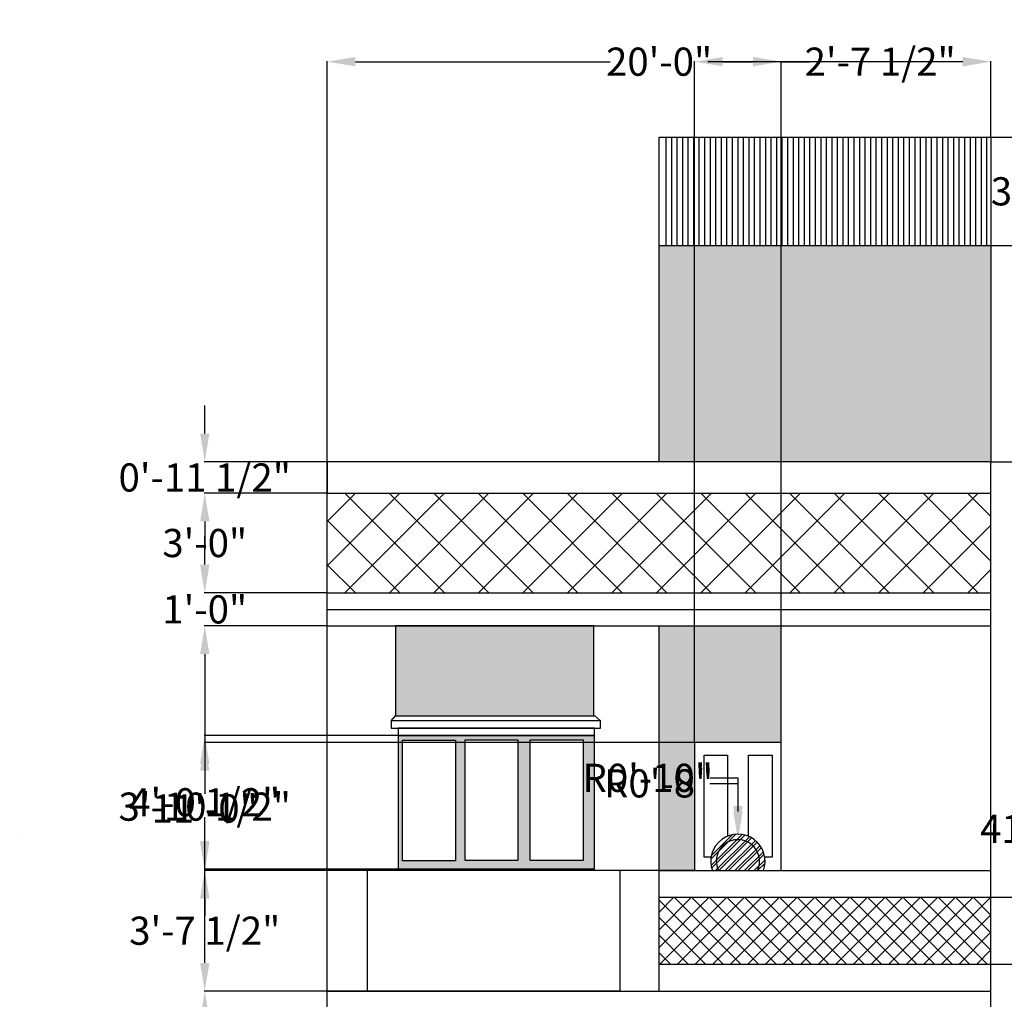
# Model space of a CAD drawing. Units: inches. Extents: x 21 to 3450, y 4 to 2137.
# Tile 6 of 14: x 2075 to 2431, y 1783 to 2137. Entities that reach past the tile are written whole.
import ezdxf

# ---------------------------------------------------------------- set-up
doc = ezdxf.new("R2010")
doc.units = ezdxf.units.IN
doc.header["$MEASUREMENT"] = 0
for name, color, linetype, lineweight in [('A-ANNO-DIMS', 2, 'Continuous', 18), ('A-ELEV', 7, 'Continuous', 25), ('A-ELEV-PATT', 8, 'Continuous', 13)]:
    doc.layers.add(name, color=color, linetype=linetype, lineweight=lineweight)
doc.styles.get("Standard").update_dxf_attribs({"font": 'arial.ttf'})
doc.dimstyles.get("Standard").update_dxf_attribs({"dimtxt": 10.18, "dimasz": 10.18, "dimexe": 0.18, "dimexo": 0.0625, "dimgap": 0.09, "dimtad": 0, "dimtih": 1, "dimtoh": 1, "dimdec": 0, "dimzin": 0, "dimdsep": 46, "dimlunit": 3, "dimtxsty": 'Standard', "dimcen": 0.09, "dimadec": 0, "dimazin": 0, "dimtfac": 1, "dimtdec": 0, "dimtofl": 0, "dimtmove": 0, "dimatfit": 3, "dimfxl": 1, "dimtolj": 1, "dimtzin": 0, "dimarcsym": 0})

# ---------------------------------------------------------------- blocks, each defined once
blk = doc.blocks.new('*D151')
at = {"layer": 'A-ANNO-DIMS', "color": 0, "lineweight": -2, "transparency": 16777216}
for p, q in [((2186.18, 1977.55), (2186.18, 2122.33)), ((2196.36, 2122.15), (2288.52, 2122.15)), ((2416, 2122.15), (2323.85, 2122.15)), ((2426.18, 2094.96), (2426.18, 2122.33))]:
    blk.add_line(p, q, dxfattribs=at)
at = {"layer": 'A-ANNO-DIMS', "color": 0, "transparency": 16777216}
for points in [[(2196.36, 2123.85), (2196.36, 2120.46), (2186.18, 2122.15)], [(2416, 2123.85), (2416, 2120.46), (2426.18, 2122.15)]]:
    blk.add_solid(points, dxfattribs=at)
at = {"layer": 'Defpoints', "color": 0, "transparency": 16777216}
for p in [(2426.18, 2122.15), (2426.18, 2094.9), (2186.18, 1977.49)]:
    blk.add_point(p, dxfattribs=at)
at = {"layer": 'A-ANNO-DIMS', "color": 0, "transparency": 16777216, "insert": (2306.18, 2122.15), "char_height": 10.18, "attachment_point": 5}
blk.add_mtext('\\A1;20\'-0"', dxfattribs=at)
blk = doc.blocks.new('*D152')
at = {"layer": 'A-ANNO-DIMS', "color": 0, "lineweight": -2, "transparency": 16777216}
for p, q in [((2426.25, 2094.9), (2453.61, 2094.9)), ((2453.43, 2084.72), (2453.43, 1850.06)), ((2453.43, 1604.7), (2453.43, 1839.36)), ((2426.25, 1594.52), (2453.61, 1594.52))]:
    blk.add_line(p, q, dxfattribs=at)
at = {"layer": 'A-ANNO-DIMS', "color": 0, "transparency": 16777216}
for points in [[(2451.74, 2084.72), (2455.13, 2084.72), (2453.43, 2094.9)], [(2451.74, 1604.7), (2455.13, 1604.7), (2453.43, 1594.52)]]:
    blk.add_solid(points, dxfattribs=at)
at = {"layer": 'Defpoints', "color": 0, "transparency": 16777216}
for p in [(2426.18, 2094.9), (2453.43, 2094.9), (2426.18, 1594.52)]:
    blk.add_point(p, dxfattribs=at)
at = {"layer": 'A-ANNO-DIMS', "color": 0, "transparency": 16777216, "insert": (2453.43, 1844.71), "char_height": 10.18, "attachment_point": 5}
blk.add_mtext('\\A1;41\'-8 1/2"', dxfattribs=at)
blk = doc.blocks.new('*D154')
at = {"layer": 'A-ANNO-DIMS', "color": 0, "lineweight": -2, "transparency": 16777216}
for p, q in [((2186.12, 1786.08), (2141.7, 1786.08)), ((2141.88, 1775.9), (2141.88, 1716.37)), ((2141.88, 1646.26), (2141.88, 1705.79)), ((2186.12, 1636.08), (2141.7, 1636.08))]:
    blk.add_line(p, q, dxfattribs=at)
at = {"layer": 'A-ANNO-DIMS', "color": 0, "transparency": 16777216}
for points in [[(2140.19, 1775.9), (2143.58, 1775.9), (2141.88, 1786.08)], [(2140.19, 1646.26), (2143.58, 1646.26), (2141.88, 1636.08)]]:
    blk.add_solid(points, dxfattribs=at)
at = {"layer": 'Defpoints', "color": 0, "transparency": 16777216}
for p in [(2141.88, 1786.08), (2186.18, 1786.08), (2186.18, 1636.08)]:
    blk.add_point(p, dxfattribs=at)
at = {"layer": 'A-ANNO-DIMS', "color": 0, "transparency": 16777216, "insert": (2141.88, 1711.08), "char_height": 10.18, "attachment_point": 5}
blk.add_mtext('\\A1;12\'-6"', dxfattribs=at)
blk = doc.blocks.new('*D155')
at = {"layer": 'A-ANNO-DIMS', "color": 0, "lineweight": -2, "transparency": 16777216}
for p, q in [((2186.12, 1918.08), (2141.7, 1918.08)), ((2141.88, 1907.9), (2141.88, 1857.37)), ((2141.88, 1796.26), (2141.88, 1846.79)), ((2186.12, 1786.08), (2141.7, 1786.08))]:
    blk.add_line(p, q, dxfattribs=at)
at = {"layer": 'A-ANNO-DIMS', "color": 0, "transparency": 16777216}
for points in [[(2140.19, 1907.9), (2143.58, 1907.9), (2141.88, 1918.08)], [(2140.19, 1796.26), (2143.58, 1796.26), (2141.88, 1786.08)]]:
    blk.add_solid(points, dxfattribs=at)
at = {"layer": 'Defpoints', "color": 0, "transparency": 16777216}
for p in [(2141.88, 1918.08), (2186.18, 1918.08), (2186.18, 1786.08)]:
    blk.add_point(p, dxfattribs=at)
at = {"layer": 'A-ANNO-DIMS', "color": 0, "transparency": 16777216, "insert": (2141.88, 1852.08), "char_height": 10.18, "attachment_point": 5}
blk.add_mtext('\\A1;11\'-0"', dxfattribs=at)
blk = doc.blocks.new('*D156')
at = {"layer": 'A-ANNO-DIMS', "color": 0, "lineweight": -2, "transparency": 16777216}
for p, q in [((2141.88, 1940.26), (2141.88, 1950.44)), ((2186.12, 1930.08), (2141.7, 1930.08)), ((2186.12, 1918.08), (2141.7, 1918.08)), ((2141.88, 1907.9), (2141.88, 1897.72))]:
    blk.add_line(p, q, dxfattribs=at)
at = {"layer": 'A-ANNO-DIMS', "color": 0, "transparency": 16777216}
for points in [[(2140.19, 1940.26), (2143.58, 1940.26), (2141.88, 1930.08)], [(2140.19, 1907.9), (2143.58, 1907.9), (2141.88, 1918.08)]]:
    blk.add_solid(points, dxfattribs=at)
at = {"layer": 'Defpoints', "color": 0, "transparency": 16777216}
for p in [(2141.88, 1930.08), (2186.18, 1930.08), (2186.18, 1918.08)]:
    blk.add_point(p, dxfattribs=at)
at = {"layer": 'A-ANNO-DIMS', "color": 0, "transparency": 16777216, "insert": (2141.88, 1924.08), "char_height": 10.18, "attachment_point": 5}
blk.add_mtext('\\A1;1\'-0"', dxfattribs=at)
blk = doc.blocks.new('*D157')
at = {"layer": 'A-ANNO-DIMS', "color": 0, "lineweight": -2, "transparency": 16777216}
for p, q in [((2186.12, 1966.08), (2141.7, 1966.08)), ((2141.88, 1955.9), (2141.88, 1953.37)), ((2141.88, 1940.26), (2141.88, 1942.79)), ((2186.12, 1930.08), (2141.7, 1930.08))]:
    blk.add_line(p, q, dxfattribs=at)
at = {"layer": 'A-ANNO-DIMS', "color": 0, "transparency": 16777216}
for points in [[(2140.19, 1955.9), (2143.58, 1955.9), (2141.88, 1966.08)], [(2140.19, 1940.26), (2143.58, 1940.26), (2141.88, 1930.08)]]:
    blk.add_solid(points, dxfattribs=at)
at = {"layer": 'Defpoints', "color": 0, "transparency": 16777216}
for p in [(2141.88, 1966.08), (2186.18, 1966.08), (2186.18, 1930.08)]:
    blk.add_point(p, dxfattribs=at)
at = {"layer": 'A-ANNO-DIMS', "color": 0, "transparency": 16777216, "insert": (2141.88, 1948.08), "char_height": 10.18, "attachment_point": 5}
blk.add_mtext('\\A1;3\'-0"', dxfattribs=at)
blk = doc.blocks.new('*D158')
at = {"layer": 'A-ANNO-DIMS', "color": 0, "lineweight": -2, "transparency": 16777216}
for p, q in [((2141.88, 1987.67), (2141.88, 1997.85)), ((2186.12, 1977.49), (2141.7, 1977.49)), ((2186.12, 1966.08), (2141.7, 1966.08)), ((2141.88, 1955.9), (2141.88, 1945.72))]:
    blk.add_line(p, q, dxfattribs=at)
at = {"layer": 'A-ANNO-DIMS', "color": 0, "transparency": 16777216}
for points in [[(2140.19, 1987.67), (2143.58, 1987.67), (2141.88, 1977.49)], [(2140.19, 1955.9), (2143.58, 1955.9), (2141.88, 1966.08)]]:
    blk.add_solid(points, dxfattribs=at)
at = {"layer": 'Defpoints', "color": 0, "transparency": 16777216}
for p in [(2141.88, 1977.49), (2186.18, 1977.49), (2186.18, 1966.08)]:
    blk.add_point(p, dxfattribs=at)
at = {"layer": 'A-ANNO-DIMS', "color": 0, "transparency": 16777216, "insert": (2141.88, 1971.78), "char_height": 10.18, "attachment_point": 5}
blk.add_mtext('\\A1;0\'-11 1/2"', dxfattribs=at)
blk = doc.blocks.new('*D159')
at = {"layer": 'A-ANNO-DIMS', "color": 0, "lineweight": -2, "transparency": 16777216}
for p, q in [((2426.25, 2055.62), (2453.61, 2055.62)), ((2453.43, 2045.44), (2453.43, 2021.84)), ((2453.43, 1987.67), (2453.43, 2011.27)), ((2426.25, 1977.49), (2453.61, 1977.49))]:
    blk.add_line(p, q, dxfattribs=at)
at = {"layer": 'A-ANNO-DIMS', "color": 0, "transparency": 16777216}
for points in [[(2451.74, 2045.44), (2455.13, 2045.44), (2453.43, 2055.62)], [(2451.74, 1987.67), (2455.13, 1987.67), (2453.43, 1977.49)]]:
    blk.add_solid(points, dxfattribs=at)
at = {"layer": 'Defpoints', "color": 0, "transparency": 16777216}
for p in [(2426.18, 2055.62), (2453.43, 2055.62), (2426.18, 1977.49)]:
    blk.add_point(p, dxfattribs=at)
at = {"layer": 'A-ANNO-DIMS', "color": 0, "transparency": 16777216, "insert": (2453.43, 2016.55), "char_height": 10.18, "attachment_point": 5}
blk.add_mtext('\\A1;6\'-6"', dxfattribs=at)
blk = doc.blocks.new('*D160')
at = {"layer": 'A-ANNO-DIMS', "color": 0, "lineweight": -2, "transparency": 16777216}
for p, q in [((2426.25, 2094.9), (2453.61, 2094.9)), ((2453.43, 2084.72), (2453.43, 2080.62)), ((2453.43, 2065.8), (2453.43, 2069.91)), ((2426.25, 2055.62), (2453.61, 2055.62))]:
    blk.add_line(p, q, dxfattribs=at)
at = {"layer": 'A-ANNO-DIMS', "color": 0, "transparency": 16777216}
for points in [[(2451.74, 2084.72), (2455.13, 2084.72), (2453.43, 2094.9)], [(2451.74, 2065.8), (2455.13, 2065.8), (2453.43, 2055.62)]]:
    blk.add_solid(points, dxfattribs=at)
at = {"layer": 'Defpoints', "color": 0, "transparency": 16777216}
for p in [(2426.18, 2094.9), (2453.43, 2094.9), (2426.18, 2055.62)]:
    blk.add_point(p, dxfattribs=at)
at = {"layer": 'A-ANNO-DIMS', "color": 0, "transparency": 16777216, "insert": (2453.43, 2075.26), "char_height": 10.18, "attachment_point": 5}
blk.add_mtext('\\A1;3\'-3 1/2"', dxfattribs=at)
blk = doc.blocks.new('*D171')
at = {"layer": 'A-ANNO-DIMS', "color": 0, "lineweight": -2, "transparency": 16777216}
for p, q in [((2282.78, 1878.5), (2141.7, 1878.5)), ((2141.88, 1868.32), (2141.88, 1859.68)), ((2141.88, 1840.33), (2141.88, 1848.97)), ((2282.78, 1830.15), (2141.7, 1830.15))]:
    blk.add_line(p, q, dxfattribs=at)
at = {"layer": 'A-ANNO-DIMS', "color": 0, "transparency": 16777216}
for points in [[(2140.19, 1868.32), (2143.58, 1868.32), (2141.88, 1878.5)], [(2140.19, 1840.33), (2143.58, 1840.33), (2141.88, 1830.15)]]:
    blk.add_solid(points, dxfattribs=at)
at = {"layer": 'Defpoints', "color": 0, "transparency": 16777216}
for p in [(2141.88, 1878.5), (2282.84, 1878.5), (2282.84, 1830.15)]:
    blk.add_point(p, dxfattribs=at)
at = {"layer": 'A-ANNO-DIMS', "color": 0, "transparency": 16777216, "insert": (2141.88, 1854.33), "char_height": 10.18, "attachment_point": 5}
blk.add_mtext('\\A1;4\'-0 1/2"', dxfattribs=at)
blk = doc.blocks.new('*D172')
at = {"layer": 'A-ANNO-DIMS', "color": 0, "lineweight": -2, "transparency": 16777216}
for p, q in [((2292.04, 1829.69), (2141.7, 1829.69)), ((2141.88, 1819.51), (2141.88, 1813.24)), ((2141.88, 1796.26), (2141.88, 1802.53)), ((2292.04, 1786.08), (2141.7, 1786.08))]:
    blk.add_line(p, q, dxfattribs=at)
at = {"layer": 'A-ANNO-DIMS', "color": 0, "transparency": 16777216}
for points in [[(2140.19, 1819.51), (2143.58, 1819.51), (2141.88, 1829.69)], [(2140.19, 1796.26), (2143.58, 1796.26), (2141.88, 1786.08)]]:
    blk.add_solid(points, dxfattribs=at)
at = {"layer": 'Defpoints', "color": 0, "transparency": 16777216}
for p in [(2141.88, 1829.69), (2292.1, 1829.69), (2292.1, 1786.08)]:
    blk.add_point(p, dxfattribs=at)
at = {"layer": 'A-ANNO-DIMS', "color": 0, "transparency": 16777216, "insert": (2141.88, 1807.89), "char_height": 10.18, "attachment_point": 5}
blk.add_mtext('\\A1;3\'-7 1/2"', dxfattribs=at)
blk = doc.blocks.new('*D174')
at = {"layer": 'A-ANNO-DIMS', "color": 0, "lineweight": -2, "transparency": 16777216}
for p, q in [((2319, 1875.96), (2319, 2122.33)), ((2329.18, 2122.15), (2340.18, 2122.15)), ((2350.36, 1875.96), (2350.36, 2122.33)), ((2350.36, 2122.15), (2360.54, 2122.15))]:
    blk.add_line(p, q, dxfattribs=at)
at = {"layer": 'A-ANNO-DIMS', "color": 0, "transparency": 16777216}
for points in [[(2329.18, 2123.85), (2329.18, 2120.46), (2319, 2122.15)], [(2340.18, 2123.85), (2340.18, 2120.46), (2350.36, 2122.15)]]:
    blk.add_solid(points, dxfattribs=at)
at = {"layer": 'Defpoints', "color": 0, "transparency": 16777216}
for p in [(2350.36, 2122.15), (2319, 1875.89), (2350.36, 1875.89)]:
    blk.add_point(p, dxfattribs=at)
at = {"layer": 'A-ANNO-DIMS', "color": 0, "transparency": 16777216, "insert": (2386.11, 2122.15), "char_height": 10.18, "attachment_point": 5}
blk.add_mtext('\\A1;2\'-7 1/2"', dxfattribs=at)
blk = doc.blocks.new('*D175')
at = {"layer": 'A-ANNO-DIMS', "color": 0, "lineweight": -2, "transparency": 16777216}
for p, q in [((2318.94, 1875.89), (2141.7, 1875.89)), ((2141.88, 1865.71), (2141.88, 1858.1)), ((2141.88, 1839.78), (2141.88, 1847.39)), ((2318.94, 1829.6), (2141.7, 1829.6))]:
    blk.add_line(p, q, dxfattribs=at)
at = {"layer": 'A-ANNO-DIMS', "color": 0, "transparency": 16777216}
for points in [[(2140.19, 1865.71), (2143.58, 1865.71), (2141.88, 1875.89)], [(2140.19, 1839.78), (2143.58, 1839.78), (2141.88, 1829.6)]]:
    blk.add_solid(points, dxfattribs=at)
at = {"layer": 'Defpoints', "color": 0, "transparency": 16777216}
for p in [(2141.88, 1875.89), (2319, 1875.89), (2319, 1829.6)]:
    blk.add_point(p, dxfattribs=at)
at = {"layer": 'A-ANNO-DIMS', "color": 0, "transparency": 16777216, "insert": (2141.88, 1852.75), "char_height": 10.18, "attachment_point": 5}
blk.add_mtext('\\A1;3\'-10 1/2"', dxfattribs=at)
blk = doc.blocks.new('*D176')
at = {"layer": 'A-ANNO-DIMS', "color": 0, "lineweight": -2, "transparency": 16777216}
for p, q in [((2453.43, 1819.97), (2453.43, 1830.15)), ((2453.43, 1830.15), (2463.61, 1830.15)), ((2306.25, 1819.97), (2453.61, 1819.97)), ((2453.43, 1805.98), (2453.43, 1809.79)), ((2306.25, 1795.8), (2453.61, 1795.8))]:
    blk.add_line(p, q, dxfattribs=at)
at = {"layer": 'A-ANNO-DIMS', "color": 0, "transparency": 16777216}
for points in [[(2451.74, 1809.79), (2455.13, 1809.79), (2453.43, 1819.97)], [(2451.74, 1805.98), (2455.13, 1805.98), (2453.43, 1795.8)]]:
    blk.add_solid(points, dxfattribs=at)
at = {"layer": 'Defpoints', "color": 0, "transparency": 16777216}
for p in [(2306.18, 1819.97), (2453.43, 1819.97), (2306.18, 1795.8)]:
    blk.add_point(p, dxfattribs=at)
at = {"layer": 'A-ANNO-DIMS', "color": 0, "transparency": 16777216, "insert": (2477.32, 1830.15), "char_height": 10.18, "attachment_point": 5}
blk.add_mtext('\\A1;2\'-0"', dxfattribs=at)
blk = doc.blocks.new('*D197')
at = {"layer": 'A-ANNO-DIMS', "color": 0, "lineweight": -2, "transparency": 16777216}
for p, q in [((2324.5, 1863.17), (2334.68, 1863.17)), ((2334.68, 1863.17), (2334.68, 1852.99)), ((2334.59, 1832.98), (2334.77, 1832.98)), ((2334.68, 1832.89), (2334.68, 1833.07))]:
    blk.add_line(p, q, dxfattribs=at)
at = {"layer": 'A-ANNO-DIMS', "color": 0, "transparency": 16777216}
blk.add_solid([(2336.38, 1852.99), (2332.99, 1852.99), (2334.68, 1842.81)], dxfattribs=at)
at = {"layer": 'Defpoints', "color": 0, "transparency": 16777216}
for p in [(2334.68, 1842.81), (2334.68, 1832.98)]:
    blk.add_point(p, dxfattribs=at)
at = {"layer": 'A-ANNO-DIMS', "color": 0, "transparency": 16777216, "insert": (2302.06, 1863.17), "char_height": 10.18, "attachment_point": 5}
blk.add_mtext('\\A1;R0\'-10"', dxfattribs=at)
blk = doc.blocks.new('*D198')
at = {"layer": 'A-ANNO-DIMS', "color": 0, "lineweight": -2, "transparency": 16777216}
for p, q in [((2324.5, 1861.17), (2334.68, 1861.17)), ((2334.68, 1861.17), (2334.68, 1850.99)), ((2334.59, 1832.98), (2334.77, 1832.98)), ((2334.68, 1832.89), (2334.68, 1833.07))]:
    blk.add_line(p, q, dxfattribs=at)
at = {"layer": 'A-ANNO-DIMS', "color": 0, "transparency": 16777216}
blk.add_solid([(2336.38, 1850.99), (2332.99, 1850.99), (2334.68, 1840.81)], dxfattribs=at)
at = {"layer": 'Defpoints', "color": 0, "transparency": 16777216}
for p in [(2334.68, 1840.81), (2334.68, 1832.98)]:
    blk.add_point(p, dxfattribs=at)
at = {"layer": 'A-ANNO-DIMS', "color": 0, "transparency": 16777216, "insert": (2306.01, 1861.17), "char_height": 10.18, "attachment_point": 5}
blk.add_mtext('\\A1;R0\'-8"', dxfattribs=at)

msp = doc.modelspace()

# ---------------------------------------------------------------- hatches: boundary and pattern name
at = {"layer": 'A-ELEV-PATT'}
h = msp.add_hatch(dxfattribs=at)
h.set_pattern_fill('AR-BRELM', color=256, scale=1.9)
h.set_pattern_definition([(0, (0, 0), (0, 10.1346), [14.4875, -0.7125]), (0, (0, 4.275), (0, 10.1346), [14.4875, -0.7125]), (0, (3.8, 5.067), (0, 10.1346), [6.8875, -0.7125]), (0, (3.8, 9.342), (0, 10.1346), [6.8875, -0.7125]), (90, (0, 0), (-15.2, 9e-16), [4.275, -5.8596]), (90, (-0.713, 0), (-15.2, 9e-16), [4.275, -5.8596]), (90, (3.8, 5.067), (-7.6, 5e-16), [4.275, -5.8596]), (90, (3.0875, 5.067), (-7.6, 5e-16), [4.275, -5.8596])])
h.paths.add_polyline_path([(2282.59, 1918.08), (2210.89, 1918.08), (2210.89, 1885.65), (2282.59, 1885.65)])
h.paths.add_polyline_path([(2280.2, 1780.08), (2208.3, 1780.08), (2208.3, 1731.04), (2280.2, 1731.04)])
h.paths.add_polyline_path([(2350.36, 1918.08), (2306.18, 1918.08), (2306.18, 1829.6), (2319, 1829.6), (2319, 1875.89), (2350.36, 1875.89)])
h.paths.add_polyline_path([(2426.18, 1780.08), (2306.18, 1780.08), (2306.18, 1636.08), (2314.57, 1636.08), (2314.57, 1734.1), (2310.48, 1734.1), (2310.48, 1737.04), (2318.62, 1741.75), (2373, 1741.75), (2378.02, 1737.04), (2378.02, 1734.1), (2374.7, 1734.1), (2374.7, 1636.08), (2384.8, 1636.08), (2384.8, 1734.1), (2382.71, 1734.1), (2382.71, 1737.37), (2387.22, 1741.92), (2420.14, 1741.92), (2422.71, 1737.37), (2422.71, 1734.1), (2420.5, 1734.1), (2420.5, 1636.08), (2426.18, 1636.08)])
h.paths.add_polyline_path([(2426.18, 2055.62), (2306.18, 2055.62), (2306.18, 1977.49), (2426.18, 1977.49)])
h = msp.add_hatch(dxfattribs=at)
h.set_pattern_fill('ANSI37', color=256, scale=91)
h.set_pattern_definition([(45, (256, -6.486), (-8.04334, 8.04334), []), (135, (256, -6.486), (-8.04334, -8.04334), [])])
h.paths.add_polyline_path([(2186.18, 1966.08), (2186.18, 1930.08), (2426.18, 1930.08), (2426.18, 1966.08)])
h = msp.add_hatch(color=256, dxfattribs=at)
h.dxf.hatch_style = 1
h.paths.add_polyline_path([(2211.87, 1878.5), (2211.87, 1830.15), (2282.84, 1830.15), (2282.84, 1878.5)])
h.paths.add_polyline_path([(2236.02, 1876.89), (2255.15, 1876.89), (2255.15, 1833.23), (2236.02, 1833.23)], flags=16)
h.paths.add_polyline_path([(2232.51, 1833.13), (2213.38, 1833.13), (2213.38, 1876.79), (2232.51, 1876.79)], flags=16)
h.paths.add_polyline_path([(2259.59, 1876.89), (2278.72, 1876.89), (2278.72, 1833.23), (2259.59, 1833.23)], flags=16)
h = msp.add_hatch(dxfattribs=at)
h.set_pattern_fill('ANSI32', color=256, scale=6.6)
h.set_pattern_definition([(45, (255.9994, -6.4862), (-1.7500893, 1.7500893), []), (45, (257.1662, -6.4862), (-1.7500893, 1.7500893), [])])
h.paths.add_polyline_path([(2327.62, 1829.6), (2341.75, 1829.6, 1.586624)], flags=17)
h.paths.add_polyline_path([(2325.45, 1829.6), (2327.62, 1829.6, -1.586624), (2341.75, 1829.6), (2343.92, 1829.6, 1.430783)])
h = msp.add_hatch(dxfattribs=at)
h.set_pattern_fill('ANSI37', color=256, scale=36)
h.set_pattern_definition([(45, (255.9994, -6.486), (-3.1819805, 3.1819805), []), (135, (255.9994, -6.486), (-3.1819805, -3.1819805), [])])
h.paths.add_polyline_path([(2426.18, 1795.8), (2426.18, 1819.97), (2306.18, 1819.97), (2306.18, 1795.8)])

# ---------------------------------------------------------------- linework, layer by layer
at = {"layer": 'A-ELEV'}
for p, q in [((2306.18, 1977.49), (2306.18, 2094.9)), ((2306.18, 2094.9), (2426.18, 2094.9)), ((2308.6, 2094.9), (2308.6, 2055.62)), ((2310.6, 2094.9), (2310.6, 2055.62)), ((2312.6, 2094.9), (2312.6, 2055.62)), ((2314.6, 2094.9), (2314.6, 2055.62)), ((2316.6, 2094.9), (2316.6, 2055.62)), ((2318.6, 2094.9), (2318.6, 2055.62)), ((2320.6, 2094.9), (2320.6, 2055.62)), ((2322.6, 2094.9), (2322.6, 2055.62)), ((2324.6, 2094.9), (2324.6, 2055.62)), ((2326.6, 2094.9), (2326.6, 2055.62)), ((2328.6, 2094.9), (2328.6, 2055.62)), ((2330.6, 2094.9), (2330.6, 2055.62)), ((2332.6, 2094.9), (2332.6, 2055.62)), ((2334.6, 2094.9), (2334.6, 2055.62)), ((2336.6, 2094.9), (2336.6, 2055.62)), ((2338.6, 2094.9), (2338.6, 2055.62)), ((2340.6, 2094.9), (2340.6, 2055.62)), ((2342.6, 2094.9), (2342.6, 2055.62)), ((2344.6, 2094.9), (2344.6, 2055.62)), ((2346.6, 2094.9), (2346.6, 2055.62)), ((2348.6, 2094.9), (2348.6, 2055.62)), ((2350.6, 2094.9), (2350.6, 2055.62)), ((2352.6, 2094.9), (2352.6, 2055.62)), ((2354.6, 2094.9), (2354.6, 2055.62)), ((2356.6, 2094.9), (2356.6, 2055.62)), ((2358.6, 2094.9), (2358.6, 2055.62)), ((2360.6, 2094.9), (2360.6, 2055.62)), ((2362.6, 2094.9), (2362.6, 2055.62)), ((2364.6, 2094.9), (2364.6, 2055.62)), ((2366.6, 2094.9), (2366.6, 2055.62)), ((2368.6, 2094.9), (2368.6, 2055.62)), ((2370.6, 2094.9), (2370.6, 2055.62)), ((2372.6, 2094.9), (2372.6, 2055.62)), ((2374.6, 2094.9), (2374.6, 2055.62)), ((2376.6, 2094.9), (2376.6, 2055.62)), ((2378.6, 2094.9), (2378.6, 2055.62)), ((2380.6, 2094.9), (2380.6, 2055.62)), ((2382.6, 2094.9), (2382.6, 2055.62)), ((2384.6, 2094.9), (2384.6, 2055.62)), ((2386.6, 2094.9), (2386.6, 2055.62)), ((2388.6, 2094.9), (2388.6, 2055.62)), ((2390.6, 2094.9), (2390.6, 2055.62)), ((2392.6, 2094.9), (2392.6, 2055.62)), ((2394.6, 2094.9), (2394.6, 2055.62)), ((2396.6, 2094.9), (2396.6, 2055.62)), ((2398.6, 2094.9), (2398.6, 2055.62)), ((2400.6, 2094.9), (2400.6, 2055.62)), ((2402.6, 2094.9), (2402.6, 2055.62)), ((2404.6, 2094.9), (2404.6, 2055.62)), ((2406.6, 2094.9), (2406.6, 2055.62)), ((2408.6, 2094.9), (2408.6, 2055.62)), ((2410.6, 2094.9), (2410.6, 2055.62)), ((2412.6, 2094.9), (2412.6, 2055.62)), ((2414.6, 2094.9), (2414.6, 2055.62)), ((2416.6, 2094.9), (2416.6, 2055.62)), ((2418.6, 2094.9), (2418.6, 2055.62)), ((2420.6, 2094.9), (2420.6, 2055.62)), ((2422.6, 2094.9), (2422.6, 2055.62)), ((2424.6, 2094.9), (2424.6, 2055.62)), ((2426.18, 2094.9), (2426.18, 1977.49)), ((2306.18, 2055.62), (2426.18, 2055.62)), ((2186.18, 1594.52), (2186.18, 1977.49)), ((2426.18, 1594.52), (2426.18, 1977.49)), ((2186.18, 1966.08), (2426.18, 1966.08)), ((2186.18, 1930.08), (2426.18, 1930.08)), ((2186.18, 1924.08), (2426.18, 1924.08)), ((2186.18, 1786.08), (2186.18, 1918.08)), ((2186.18, 1786.08), (2186.18, 1918.08)), ((2186.18, 1918.08), (2426.18, 1918.08)), ((2306.18, 1786.08), (2306.18, 1918.08)), ((2350.36, 1875.89), (2350.36, 1918.08)), ((2209.31, 1883.78), (2210.89, 1885.65)), ((2210.89, 1885.65), (2282.91, 1885.65)), ((2284.98, 1883.78), (2282.91, 1885.65)), ((2306.18, 1829.6), (2426.18, 1829.6)), ((2426.18, 1795.8), (2426.18, 1825.1)), ((2306.18, 1819.97), (2426.18, 1819.97)), ((2306.18, 1795.8), (2426.18, 1795.8)), ((2186.18, 1786.08), (2426.18, 1786.08))]:
    msp.add_line(p, q, dxfattribs=at)
for points in [[(2186.18, 1966.08), (2186.18, 1966.08), (2426.18, 1966.08), (2426.18, 1966.08), (2426.18, 1977.49), (2426.18, 1977.49), (2186.18, 1977.49), (2186.18, 1977.49)], [(2210.89, 1885.65), (2210.89, 1885.65), (2282.59, 1885.65), (2282.59, 1885.65), (2282.59, 1918.08), (2282.59, 1918.08), (2210.89, 1918.08), (2210.89, 1918.08)], [(2209.31, 1881.09), (2209.31, 1881.09), (2284.98, 1881.09), (2284.98, 1881.09), (2284.98, 1883.78), (2284.98, 1883.78), (2209.31, 1883.78), (2209.31, 1883.78)], [(2211.87, 1878.5), (2211.87, 1878.5), (2282.79, 1878.5), (2282.79, 1878.5), (2282.79, 1881.09), (2282.79, 1881.09), (2211.87, 1881.09), (2211.87, 1881.09)], [(2211.87, 1830.15), (2211.87, 1830.15), (2282.84, 1830.15), (2282.84, 1830.15), (2282.84, 1878.5), (2282.84, 1878.5), (2211.87, 1878.5), (2211.87, 1878.5)], [(2213.38, 1876.79), (2213.38, 1876.79), (2232.51, 1876.79), (2232.51, 1876.79), (2232.51, 1833.13), (2232.51, 1833.13), (2213.38, 1833.13), (2213.38, 1833.13)], [(2236.02, 1876.89), (2236.02, 1876.89), (2255.15, 1876.89), (2255.15, 1876.89), (2255.15, 1833.23), (2255.15, 1833.23), (2236.02, 1833.23), (2236.02, 1833.23)], [(2259.59, 1876.89), (2259.59, 1876.89), (2278.72, 1876.89), (2278.72, 1876.89), (2278.72, 1833.23), (2278.72, 1833.23), (2259.59, 1833.23), (2259.59, 1833.23)], [(2319, 1829.6), (2319, 1829.6), (2350.36, 1829.6), (2350.36, 1829.6), (2350.36, 1875.89), (2350.36, 1875.89), (2319, 1875.89), (2319, 1875.89)], [(2074.96, 1840.94), (2074.96, 1840.94)], [(2200.57, 1786.08), (2200.57, 1786.08), (2292.1, 1786.08), (2292.1, 1786.08), (2292.1, 1829.69), (2292.1, 1829.69), (2200.57, 1829.69), (2200.57, 1829.69)]]:
    msp.add_lwpolyline(points, close=True, dxfattribs=at)
for points in [[(2324.96, 1834.46), (2322.42, 1834.46), (2322.42, 1834.46), (2322.42, 1871.39), (2322.42, 1871.39), (2330.96, 1871.39), (2330.96, 1871.39), (2330.96, 1842.08)], [(2338.5, 1842.04), (2338.5, 1871.39), (2338.5, 1871.39), (2347.04, 1871.39), (2347.04, 1871.39), (2347.04, 1834.46), (2347.04, 1834.46), (2344.41, 1834.46)]]:
    msp.add_lwpolyline(points, dxfattribs=at)
for radius, start, end in [(9.83, 339.9008, 200.0992), (7.83, 334.4439, 205.5561)]:
    msp.add_arc((2334.68, 1832.98), radius, start, end, dxfattribs=at)

# ---------------------------------------------------------------- dimensions: what is measured, and where the dimension line sits
at = {"layer": 'A-ANNO-DIMS'}
for base, p1, p2, picture, middle in [((2350.36, 2122.15), (2319, 1875.89), (2350.36, 1875.89), '*D174', (2386.11, 2122.15)), ((2426.18, 2122.15), (2186.18, 1977.49), (2426.18, 2094.9), '*D151', (2306.18, 2122.15))]:
    dim = msp.add_linear_dim(base=base, p1=p1, p2=p2, dimstyle='Standard', override={"dimdec": 1, "dimlfac": 1, "dimrnd": 0, "dimzin": 1, "dimdsep": 46, "dimlunit": 4, "dimfrac": 2}, dxfattribs=at)
    dim.commit()
    dim.dimension.update_dxf_attribs({"geometry": picture, "text_midpoint": middle})
for base, p1, p2, picture, middle in [((2453.43, 2094.9), (2426.18, 1594.52), (2426.18, 2094.9), '*D152', (2453.43, 1844.71)), ((2453.43, 2094.9), (2426.18, 2055.62), (2426.18, 2094.9), '*D160', (2453.43, 2075.26)), ((2453.43, 2055.62), (2426.18, 1977.49), (2426.18, 2055.62), '*D159', (2453.43, 2016.55)), ((2141.88, 1977.49), (2186.18, 1966.08), (2186.18, 1977.49), '*D158', (2141.88, 1971.78)), ((2141.88, 1966.08), (2186.18, 1930.08), (2186.18, 1966.08), '*D157', (2141.88, 1948.08)), ((2141.88, 1930.08), (2186.18, 1918.08), (2186.18, 1930.08), '*D156', (2141.88, 1924.08)), ((2141.88, 1918.08), (2186.18, 1786.08), (2186.18, 1918.08), '*D155', (2141.88, 1852.08)), ((2141.88376, 1878.50359), (2282.84041, 1830.1536), (2282.84041, 1878.50359), '*D171', (2141.88376, 1854.3286)), ((2141.88, 1875.89), (2319, 1829.6), (2319, 1875.89), '*D175', (2141.88, 1852.75)), ((2453.43, 1819.97), (2306.18, 1795.8), (2306.18, 1819.97), '*D176', (2477.32, 1830.15)), ((2141.88, 1829.69), (2292.1, 1786.08), (2292.1, 1829.69), '*D172', (2141.88, 1807.89)), ((2141.88, 1786.08), (2186.18, 1636.08), (2186.18, 1786.08), '*D154', (2141.88, 1711.08))]:
    dim = msp.add_linear_dim(base=base, p1=p1, p2=p2, angle=90, dimstyle='Standard', override={"dimdec": 1, "dimlfac": 1, "dimrnd": 0, "dimzin": 1, "dimdsep": 46, "dimlunit": 4, "dimfrac": 2}, dxfattribs=at)
    dim.commit()
    dim.dimension.update_dxf_attribs({"geometry": picture, "text_midpoint": middle})
for mpoint, picture, middle in [((2334.68, 1842.81), '*D197', (2302.06, 1863.17)), ((2334.68, 1840.81), '*D198', (2306.01, 1861.17))]:
    dim = msp.add_radius_dim(center=(2334.68, 1832.98), mpoint=mpoint, dimstyle='Standard', override={"dimdec": 1, "dimlfac": 1, "dimrnd": 0, "dimzin": 1, "dimdsep": 46, "dimlunit": 4, "dimfrac": 2}, dxfattribs=at)
    dim.commit()
    dim.dimension.update_dxf_attribs({"geometry": picture, "text_midpoint": middle})

doc.saveas('drawing.dxf')
